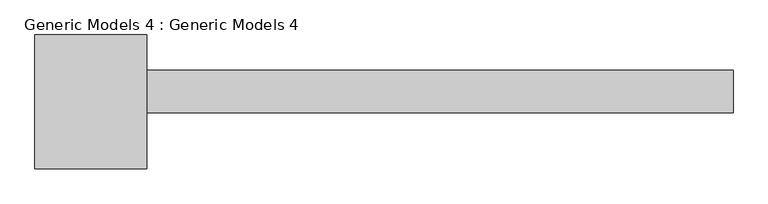
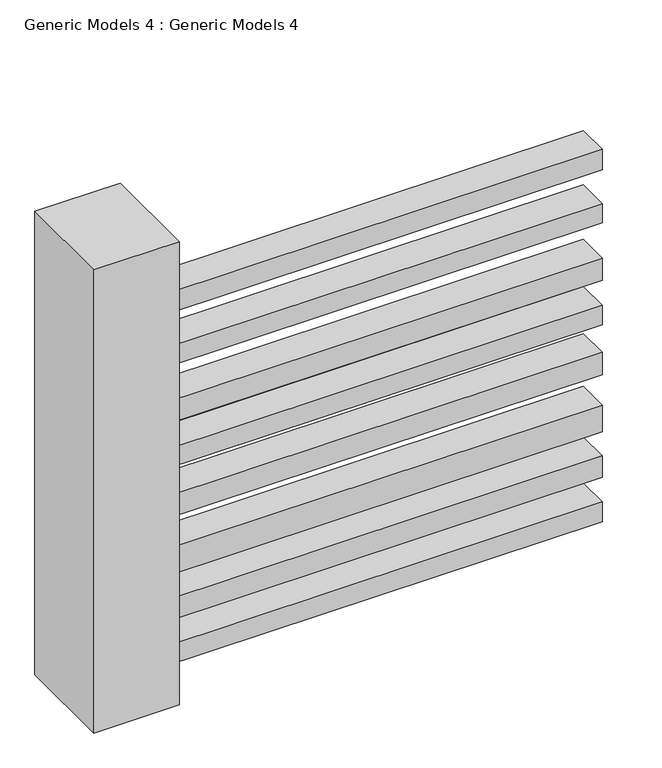
"""IFC4 building model written with IfcOpenShell, lengths in millimetres: proxy geometry, Generic Models 4 : Generic Models 4."""

from ifc_helpers import new_model, si_unit, frame, origin, place, context, project, spatial, polyline, outline, extrude, source, transform, mapped, element, save


def generic_models_4_generic_models_4_7ae05182(model_context):
    return source(origin(), model_context, "Body", "SweptSolid", [
        extrude(outline(polyline([(-3321.6830976, -12239.8345564), (-3321.6830976, -12392.2345564), (-5421.0588485, -12392.2345564), (-5421.0588485, -12239.8345564), (-3321.6830976, -12239.8345564)])), frame((0.0, 0.0, 2100.4053279), z_axis=(0.0, 0.0, 1.0), x_axis=(1.0, 0.0, 0.0)), (0.0, 0.0, 1.0), 101.6),
        extrude(outline(polyline([(-3321.6830976, -12239.8345564), (-3321.6830976, -12392.2345564), (-5421.0588485, -12392.2345564), (-5421.0588485, -12239.8345564), (-3321.6830976, -12239.8345564)])), frame((0.0, 0.0, 1838.534941), z_axis=(0.0, 0.0, 1.0), x_axis=(1.0, 0.0, 0.0)), (0.0, 0.0, 1.0), 95.3746772),
        extrude(outline(polyline([(-3321.6830976, -12239.8345564), (-3321.6830976, -12392.2345564), (-5421.0588485, -12392.2345564), (-5421.0588485, -12239.8345564), (-3321.6830976, -12239.8345564)])), frame((0.0, 0.0, 1554.7779195), z_axis=(0.0, 0.0, 1.0), x_axis=(1.0, 0.0, 0.0)), (0.0, 0.0, 1.0), 109.1490813),
        extrude(outline(polyline([(-3321.6830976, -12239.8345564), (-3321.6830976, -12392.2345564), (-5421.0588485, -12392.2345564), (-5421.0588485, -12239.8345564), (-3321.6830976, -12239.8345564)])), frame((0.0, 0.0, 1333.879396), z_axis=(0.0, 0.0, 1.0), x_axis=(1.0, 0.0, 0.0)), (0.0, 0.0, 1.0), 95.1413263),
        extrude(outline(polyline([(-3321.6830976, -12239.8345564), (-3321.6830976, -12392.2345564), (-5421.0588485, -12392.2345564), (-5421.0588485, -12239.8345564), (-3321.6830976, -12239.8345564)])), frame((0.0, 0.0, 1085.418664), z_axis=(0.0, 0.0, 1.0), x_axis=(1.0, 0.0, 0.0)), (0.0, 0.0, 1.0), 110.3158358),
        extrude(outline(polyline([(-3321.6830976, -12239.8345564), (-3321.6830976, -12392.2345564), (-5421.0588485, -12392.2345564), (-5421.0588485, -12239.8345564), (-3321.6830976, -12239.8345564)])), frame((0.0, 0.0, 801.6415419), z_axis=(0.0, 0.0, 1.0), x_axis=(1.0, 0.0, 0.0)), (0.0, 0.0, 1.0), 133.244527),
        extrude(outline(polyline([(-3321.6830976, -12239.8345564), (-3321.6830976, -12392.2345564), (-5421.0588485, -12392.2345564), (-5421.0588485, -12239.8345564), (-3321.6830976, -12239.8345564)])), frame((0.0, 0.0, 577.0228041), z_axis=(0.0, 0.0, 1.0), x_axis=(1.0, 0.0, 0.0)), (0.0, 0.0, 1.0), 105.4087665),
        extrude(outline(polyline([(-3321.6830976, -12239.8345564), (-3321.6830976, -12392.2345564), (-5421.0588485, -12392.2345564), (-5421.0588485, -12239.8345564), (-3321.6830976, -12239.8345564)])), frame((0.0, 0.0, 357.0576843), z_axis=(0.0, 0.0, 1.0), x_axis=(1.0, 0.0, 0.0)), (0.0, 0.0, 1.0), 97.9482374),
        extrude(outline(polyline([(-5820.6120831, -12113.2945627), (-5421.0588485, -12113.2945627), (-5421.0588485, -12592.2491176), (-5820.6120831, -12592.2491176), (-5820.6120831, -12113.2945627)])), frame((0.0, 0.0, 304.8), z_axis=(0.0, 0.0, 1.0), x_axis=(1.0, 0.0, 0.0)), (0.0, 0.0, 1.0), 2296.0541964),
    ])


if __name__ == "__main__":
    model = new_model("IFC4")
    model_context = context("Model", 3, world=origin())
    ifc_project = project(units=[si_unit("LENGTHUNIT", "METRE", prefix="MILLI")], contexts=[model_context])
    site = spatial("IfcSite", under=ifc_project)
    building = spatial("IfcBuilding", under=site)
    placement = place(None, origin())
    generic_models_4_generic_models_4_shape = generic_models_4_generic_models_4_7ae05182(model_context)
    element("IfcBuildingElementProxy", 1, Name="Generic Models 4 : Generic Models 4", ObjectType="Generic Models 4 : Generic Models 4", at=placement, inside=building, context=model_context, shape_type="MappedRepresentation", body=[
        mapped(generic_models_4_generic_models_4_shape, transform((0.0, 0.0, 0.0), x_axis=(1.0, 0.0, 0.0), y_axis=(0.0, 1.0, 0.0), z_axis=(0.0, 0.0, 1.0))),
    ])
    save(model, "model.ifc")
